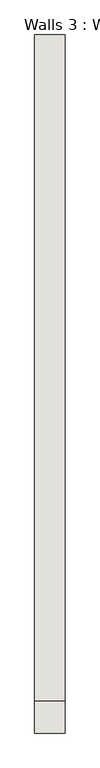
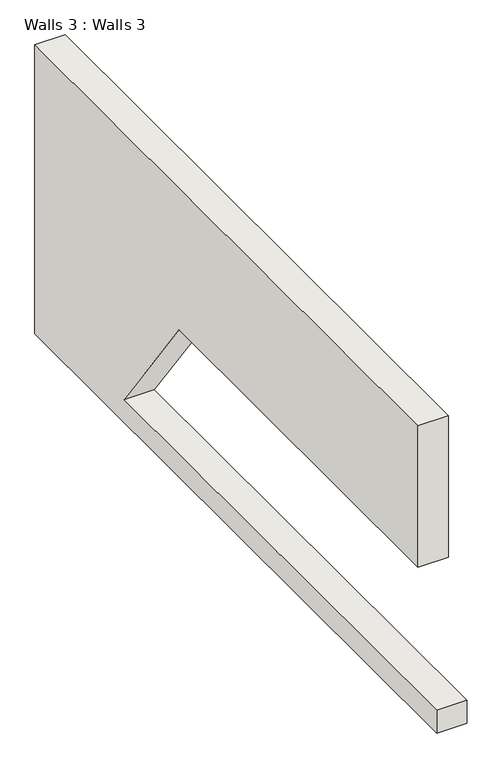
"""IFC4 building model written with IfcOpenShell, lengths in millimetres: wall geometry, Walls 3 : Walls 3."""

from ifc_helpers import new_model, si_unit, frame, origin, place, context, project, spatial, polyline, outline, extrude, source, transform, mapped, element, save


def walls_3_walls_3_cd5a9325(model_context):
    return source(origin(), model_context, "Body", "SweptSolid", [
        extrude(outline(polyline([(-9939.1578064, 2648.0), (-9939.1578064, 3048.0), (-883.6554166, 3048.0), (-2484.5555499, 5251.45), (-9401.6681843, 5251.45), (-9401.6681843, 7747.0809544), (1695.6421936, 7747.0809544), (1695.6421936, 2648.0), (-9939.1578064, 2648.0)])), frame((11635.2505118, 0.0, 0.0), z_axis=(1.0, 0.0, 0.0), x_axis=(0.0, 1.0, 0.0)), (0.0, 0.0, 1.0), 504.8),
    ])


if __name__ == "__main__":
    model = new_model("IFC4")
    model_context = context("Model", 3, world=origin())
    ifc_project = project(units=[si_unit("LENGTHUNIT", "METRE", prefix="MILLI")], contexts=[model_context])
    site = spatial("IfcSite", under=ifc_project)
    building = spatial("IfcBuilding", under=site)
    placement = place(None, origin())
    walls_3_walls_3_shape = walls_3_walls_3_cd5a9325(model_context)
    element("IfcWall", 1, ObjectType="Walls 3 : Walls 3", at=placement, inside=building, context=model_context, shape_type="MappedRepresentation", body=[
        mapped(walls_3_walls_3_shape, transform((0.0, 0.0, 0.0), x_axis=(1.0, 0.0, 0.0), y_axis=(0.0, 1.0, 0.0), z_axis=(0.0, 0.0, 1.0))),
    ])
    save(model, "model.ifc")

# Revit data of these elements
# Element 1 (IfcWall, "Walls 3 : Walls 3")
#   Materials on its faces: "Default Wall"
# Materials
#   "Default Wall": colour RGB 80 80 80, transparency 0
